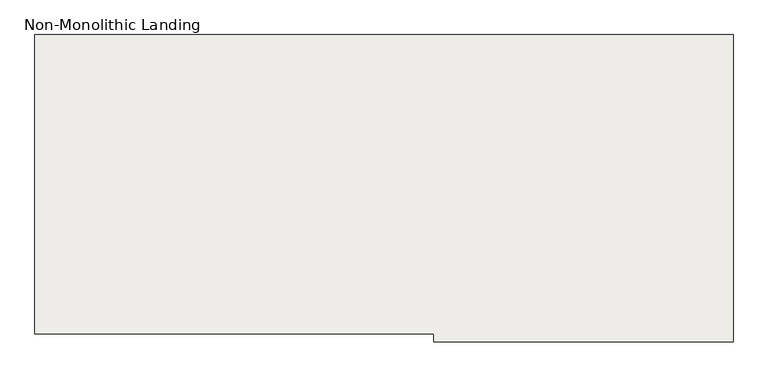
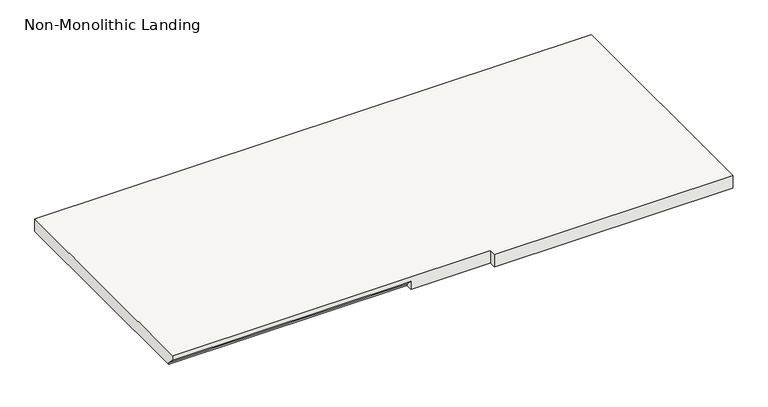
"""IFC4 building model written with IfcOpenShell, lengths in millimetres: slab geometry, Non-Monolithic Landing."""

from ifc_helpers import new_model, si_unit, origin, place, context, project, spatial, faceted_brep, source, transform, mapped, element, save


def non_monolithic_landing_cdb44c8c(model_context):
    return source(origin(), model_context, "Body", "Brep", [
        faceted_brep([(7464.4260838, 825.5660813, 1712.7681818), (7464.4260838, 850.9660813, 1687.3681818), (8378.8260838, 850.9660813, 1687.3681818), (8378.8260838, 825.5660813, 1712.7681818), (8683.6260838, 825.5660813, 1731.8181818), (8683.6260838, 800.1660813, 1731.8181818), (9598.0260838, 800.1660813, 1731.8181818), (9598.0260838, 825.5660813, 1731.8181818), (9598.0260838, 1739.9660813, 1731.8181818), (7464.4260838, 1739.9660813, 1731.8181818), (7464.4260838, 825.5660813, 1731.8181818), (8378.8260838, 850.9660813, 1681.0181818), (7464.4260838, 850.9660813, 1681.0181818), (7464.4260838, 1739.9660813, 1681.0181818), (9598.0260838, 1739.9660813, 1681.0181818), (9598.0260838, 825.5660813, 1681.0181818), (9598.0260838, 800.1660813, 1681.0181818), (8683.6260838, 800.1660813, 1681.0181818), (8683.6260838, 825.5660813, 1681.0181818), (8378.8260838, 825.5660813, 1681.0181818)], [[[0, 1, 2, 3]], [[4, 5, 6, 7, 8, 9, 10]], [[11, 12, 13, 14, 15, 16, 17, 18, 19]], [[12, 11, 2, 1]], [[11, 19, 3, 2]], [[4, 10, 0, 3, 19, 18]], [[5, 4, 18, 17]], [[6, 5, 17, 16]], [[7, 6, 16, 15]], [[8, 7, 15, 14]], [[9, 8, 14, 13]], [[10, 9, 13, 12, 1, 0]]]),
    ])


if __name__ == "__main__":
    model = new_model("IFC4")
    model_context = context("Model", 3, world=origin())
    ifc_project = project(units=[si_unit("LENGTHUNIT", "METRE", prefix="MILLI")], contexts=[model_context])
    site = spatial("IfcSite", under=ifc_project)
    building = spatial("IfcBuilding", under=site)
    placement = place(None, origin())
    non_monolithic_landing_shape = non_monolithic_landing_cdb44c8c(model_context)
    element("IfcSlab", 1, ObjectType="Non-Monolithic Landing", at=placement, inside=building, context=model_context, shape_type="MappedRepresentation", body=[
        mapped(non_monolithic_landing_shape, transform((0.0, 0.0, 0.0), x_axis=(1.0, 0.0, 0.0), y_axis=(0.0, 1.0, 0.0), z_axis=(0.0, 0.0, 1.0))),
    ])
    save(model, "model.ifc")
